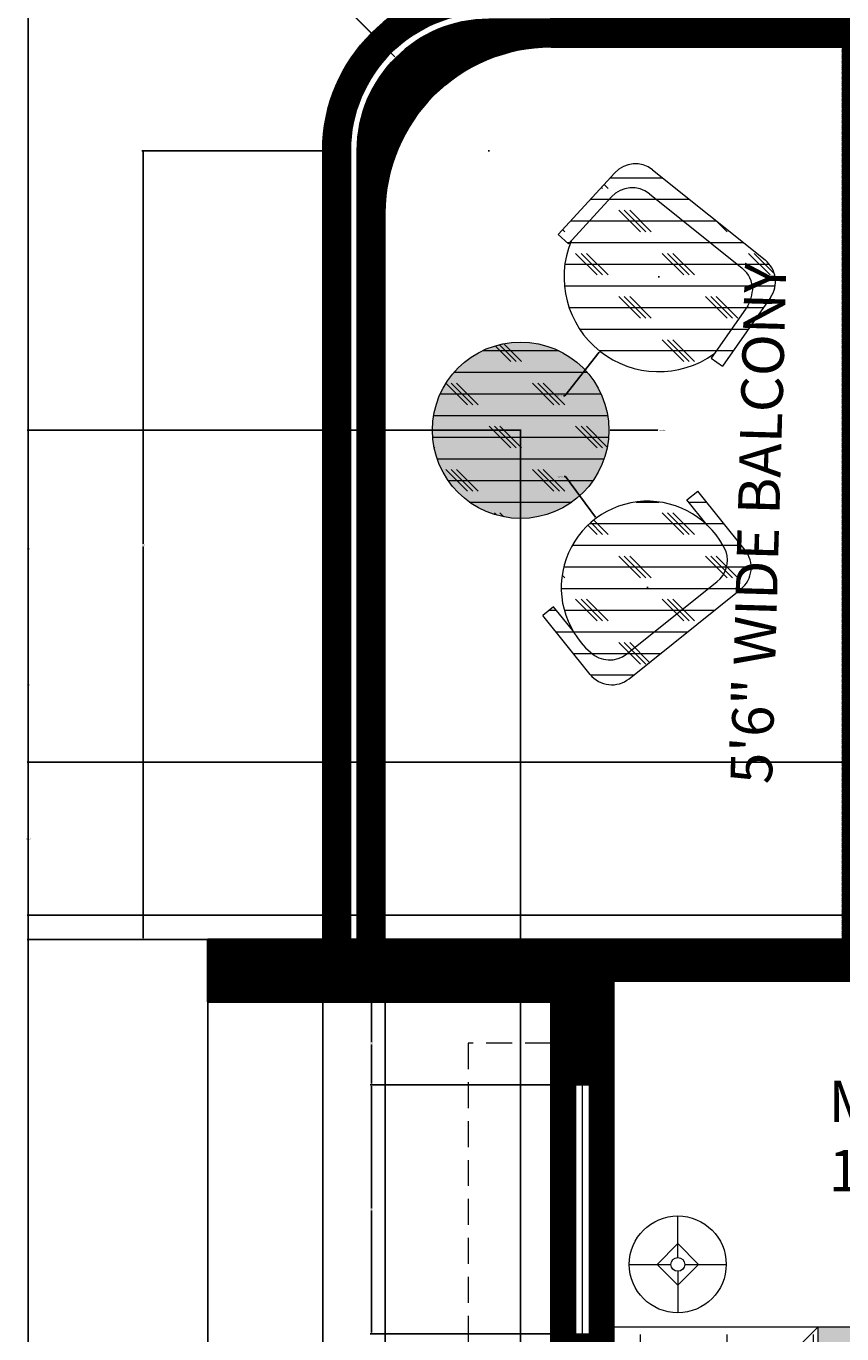
# Model space of a CAD drawing. Units: inches. Extents: x 557 to 1007, y 390 to 953.
# Tile 3 of 10: x 557 to 674, y 558 to 747. Entities that reach past the tile are written whole.
import ezdxf

# ---------------------------------------------------------------- set-up
doc = ezdxf.new("R2010")
doc.units = ezdxf.units.IN
doc.header["$LTSCALE"] = 5
doc.header["$MEASUREMENT"] = 0
doc.linetypes.add('HIDDEN', pattern=[0.375, 0.25, -0.125])
for name, color, linetype, lineweight in [('A-ANNO-DIMS', 2, 'Continuous', 18), ('A-AREA-IDEN', 7, 'Continuous', 18), ('A-FLOR-RAIL', 7, 'Continuous', 25), ('A-FURN', 8, 'Continuous', 18), ('A-FURN-PATT', 9, 'Continuous', 9), ('A-GLAZ', 4, 'Continuous', 18), ('A-GLAZ-OVHD', 8, 'HIDDEN', 13), ('A-WALL', 7, 'Continuous', 35), ('E-LITE', 2, 'Continuous', 13)]:
    doc.layers.add(name, color=color, linetype=linetype, lineweight=lineweight)
doc.layers.add('A-GLAZ-PATT', color=141, linetype='Continuous', lineweight=9, true_color=0xadddf7)
doc.layers.add('A-WALL-PATT', color=251, linetype='Continuous', lineweight=9, true_color=0x636466)
doc.styles.get("Standard").update_dxf_attribs({"font": 'arial.ttf'})
doc.dimstyles.get("Standard").update_dxf_attribs({"dimtxt": 0.18, "dimasz": 0.18, "dimexe": 0.18, "dimexo": 0.0625, "dimgap": 0.09, "dimtad": 0, "dimtih": 1, "dimtoh": 1, "dimdec": 4, "dimzin": 0, "dimdsep": 46, "dimtxsty": 'Standard', "dimcen": 0.09, "dimadec": 0, "dimazin": 0, "dimtfac": 1, "dimtdec": 4, "dimtofl": 0, "dimtmove": 0, "dimatfit": 3, "dimfxl": 1, "dimtolj": 1, "dimtzin": 0, "dimarcsym": 0})

# ---------------------------------------------------------------- blocks, each defined once
blk = doc.blocks.new('Lamp - Table')
for p, q in [((0, 7), (0, 1)), ((0, 3), (-3, 0)), ((3, 0), (0, 3)), ((-1, 0), (-7, 0)), ((-3, 0), (0, -3)), ((0, -3), (3, 0)), ((1, 0), (7, 0)), ((0, -1), (0, -7))]:
    blk.add_line(p, q)
for radius in [7, 1]:
    blk.add_circle((0, 0), radius)
blk = doc.blocks.new('BED-QUEEN-60x80-PLAN')
for p, q in [((0, 0), (0, 60)), ((0, 60), (80, 60)), ((29.6, 60), (14.4, 44.8)), ((29.6, 44.8), (29.6, 60)), ((80, 60), (80, 0)), ((1.2, 52), (16.4, 52)), ((1.2, 31.2), (1.2, 52)), ((16.4, 52), (16.4, 46.8)), ((14.4, 0), (14.4, 44.8)), ((14.4, 44.8), (29.6, 44.8)), ((16.8, 44.8), (16.8, 0)), ((14.4, 31.2), (1.2, 31.2)), ((1.2, 28.8), (14.4, 28.8)), ((1.2, 8), (1.2, 28.8)), ((14.4, 8), (1.2, 8)), ((80, 0), (0, 0))]:
    blk.add_line(p, q)
blk = doc.blocks.new('*D45')
at = {"layer": 'A-ANNO-DIMS', "color": 0, "lineweight": -2, "ltscale": 5, "transparency": 16777216}
for p, q in [((582.82, 605.84), (582.82, 389.77)), ((980.41, 439.84), (980.41, 389.77)), ((583, 389.95), (781.22, 389.95)), ((980.23, 389.95), (782.01, 389.95))]:
    blk.add_line(p, q, dxfattribs=at)
at = {"layer": 'A-ANNO-DIMS', "color": 0, "ltscale": 5, "transparency": 16777216}
for points in [[(583, 389.98), (583, 389.92), (582.82, 389.95)], [(980.23, 389.98), (980.23, 389.92), (980.41, 389.95)]]:
    blk.add_solid(points, dxfattribs=at)
at = {"layer": 'Defpoints', "color": 0, "ltscale": 5, "transparency": 16777216}
for p in [(582.82, 605.9), (980.41, 439.9), (980.41, 389.95)]:
    blk.add_point(p, dxfattribs=at)
at = {"layer": 'A-ANNO-DIMS', "color": 0, "ltscale": 5, "transparency": 16777216, "insert": (781.61, 389.95), "char_height": 0.18, "attachment_point": 5}
blk.add_mtext('\\A1;397.6', dxfattribs=at)
blk = doc.blocks.new('*D46')
at = {"layer": 'A-ANNO-DIMS', "color": 0, "lineweight": -2, "ltscale": 5, "transparency": 16777216}
for p, q in [((761.34, 926.9), (556.69, 926.9)), ((556.87, 926.72), (556.87, 671.59)), ((556.87, 416.08), (556.87, 671.22)), ((773.34, 415.9), (556.69, 415.9))]:
    blk.add_line(p, q, dxfattribs=at)
at = {"layer": 'A-ANNO-DIMS', "color": 0, "ltscale": 5, "transparency": 16777216}
for points in [[(556.84, 926.72), (556.9, 926.72), (556.87, 926.9)], [(556.84, 416.08), (556.9, 416.08), (556.87, 415.9)]]:
    blk.add_solid(points, dxfattribs=at)
at = {"layer": 'Defpoints', "color": 0, "ltscale": 5, "transparency": 16777216}
for p in [(556.87, 926.9), (761.41, 926.9), (773.41, 415.9)]:
    blk.add_point(p, dxfattribs=at)
at = {"layer": 'A-ANNO-DIMS', "color": 0, "ltscale": 5, "transparency": 16777216, "insert": (556.87, 671.4), "char_height": 0.18, "attachment_point": 5}
blk.add_mtext('\\A1;511', dxfattribs=at)
blk = doc.blocks.new('*D59')
at = {"layer": 'A-ANNO-DIMS', "color": 0, "lineweight": -2, "ltscale": 5, "transparency": 16777216}
for p, q in [((599.34, 728.9), (573.28, 728.9)), ((573.46, 728.72), (573.46, 672.08)), ((573.46, 615.08), (573.46, 671.72)), ((599.34, 614.9), (573.28, 614.9))]:
    blk.add_line(p, q, dxfattribs=at)
at = {"layer": 'A-ANNO-DIMS', "color": 0, "ltscale": 5, "transparency": 16777216}
for points in [[(573.43, 728.72), (573.49, 728.72), (573.46, 728.9)], [(573.43, 615.08), (573.49, 615.08), (573.46, 614.9)]]:
    blk.add_solid(points, dxfattribs=at)
at = {"layer": 'Defpoints', "color": 0, "ltscale": 5, "transparency": 16777216}
for p in [(573.46, 728.9), (599.41, 728.9), (599.41, 614.9)]:
    blk.add_point(p, dxfattribs=at)
at = {"layer": 'A-ANNO-DIMS', "color": 0, "ltscale": 5, "transparency": 16777216, "insert": (573.46, 671.9), "char_height": 0.18, "attachment_point": 5}
blk.add_mtext('\\A1;114', dxfattribs=at)
blk = doc.blocks.new('*D65')
at = {"layer": 'A-ANNO-DIMS', "color": 0, "lineweight": -2, "ltscale": 5, "transparency": 16777216}
for p, q in [((632.34, 593.9), (606.28, 593.9)), ((606.46, 593.72), (606.46, 576.09)), ((606.46, 558.08), (606.46, 575.72)), ((632.34, 557.9), (606.28, 557.9))]:
    blk.add_line(p, q, dxfattribs=at)
at = {"layer": 'A-ANNO-DIMS', "color": 0, "ltscale": 5, "transparency": 16777216}
for points in [[(606.43, 593.72), (606.49, 593.72), (606.46, 593.9)], [(606.43, 558.08), (606.49, 558.08), (606.46, 557.9)]]:
    blk.add_solid(points, dxfattribs=at)
at = {"layer": 'Defpoints', "color": 0, "ltscale": 5, "transparency": 16777216}
for p in [(606.46, 593.9), (632.41, 593.9), (632.41, 557.9)]:
    blk.add_point(p, dxfattribs=at)
at = {"layer": 'A-ANNO-DIMS', "color": 0, "ltscale": 5, "transparency": 16777216, "insert": (606.46, 575.9), "char_height": 0.18, "attachment_point": 5}
blk.add_mtext('\\A1;36', dxfattribs=at)
blk = doc.blocks.new('*D66')
at = {"layer": 'A-ANNO-DIMS', "color": 0, "lineweight": -2, "ltscale": 5, "transparency": 16777216}
for p, q in [((632.34, 605.9), (606.28, 605.9)), ((606.46, 605.72), (606.46, 600.08)), ((606.46, 594.08), (606.46, 599.72)), ((632.34, 593.9), (606.28, 593.9))]:
    blk.add_line(p, q, dxfattribs=at)
at = {"layer": 'A-ANNO-DIMS', "color": 0, "ltscale": 5, "transparency": 16777216}
for points in [[(606.43, 605.72), (606.49, 605.72), (606.46, 605.9)], [(606.43, 594.08), (606.49, 594.08), (606.46, 593.9)]]:
    blk.add_solid(points, dxfattribs=at)
at = {"layer": 'Defpoints', "color": 0, "ltscale": 5, "transparency": 16777216}
for p in [(606.46, 605.9), (632.41, 605.9), (632.41, 593.9)]:
    blk.add_point(p, dxfattribs=at)
at = {"layer": 'A-ANNO-DIMS', "color": 0, "ltscale": 5, "transparency": 16777216, "insert": (606.46, 599.9), "char_height": 0.18, "attachment_point": 5}
blk.add_mtext('\\A1;12', dxfattribs=at)
blk = doc.blocks.new('*D75')
at = {"layer": 'A-ANNO-DIMS', "color": 0, "lineweight": -2, "ltscale": 5, "transparency": 16777216}
for p, q in [((582.82, 614.84), (582.82, 389.77)), ((599.41, 614.84), (599.41, 389.77)), ((583, 389.95), (590.66, 389.95)), ((599.23, 389.95), (591.57, 389.95))]:
    blk.add_line(p, q, dxfattribs=at)
at = {"layer": 'A-ANNO-DIMS', "color": 0, "ltscale": 5, "transparency": 16777216}
for points in [[(583, 389.98), (583, 389.92), (582.82, 389.95)], [(599.23, 389.98), (599.23, 389.92), (599.41, 389.95)]]:
    blk.add_solid(points, dxfattribs=at)
at = {"layer": 'Defpoints', "color": 0, "ltscale": 5, "transparency": 16777216}
for p in [(582.82, 614.9), (599.41, 614.9), (582.82, 389.95)]:
    blk.add_point(p, dxfattribs=at)
at = {"layer": 'A-ANNO-DIMS', "color": 0, "ltscale": 5, "transparency": 16777216, "insert": (591.11, 389.95), "char_height": 0.18, "attachment_point": 5}
blk.add_mtext('\\A1;16.582', dxfattribs=at)
blk = doc.blocks.new('*D81')
at = {"layer": 'A-ANNO-DIMS', "color": 0, "lineweight": -2, "ltscale": 5, "transparency": 16777216}
for p, q in [((874.87, 640.54), (556.69, 640.54)), ((556.87, 640.36), (556.87, 629.66)), ((556.87, 618.59), (556.87, 629.29)), ((870.87, 618.41), (556.69, 618.41))]:
    blk.add_line(p, q, dxfattribs=at)
at = {"layer": 'A-ANNO-DIMS', "color": 0, "ltscale": 5, "transparency": 16777216}
for points in [[(556.84, 640.36), (556.9, 640.36), (556.87, 640.54)], [(556.84, 618.59), (556.9, 618.59), (556.87, 618.41)]]:
    blk.add_solid(points, dxfattribs=at)
at = {"layer": 'Defpoints', "color": 0, "ltscale": 5, "transparency": 16777216}
for p in [(874.93, 640.54), (556.87, 618.41), (870.93, 618.41)]:
    blk.add_point(p, dxfattribs=at)
at = {"layer": 'A-ANNO-DIMS', "color": 0, "ltscale": 5, "transparency": 16777216, "insert": (556.87, 629.48), "char_height": 0.18, "attachment_point": 5}
blk.add_mtext('\\A1;22.13', dxfattribs=at)
blk = doc.blocks.new('*D91')
at = {"layer": 'A-ANNO-DIMS', "color": 0, "lineweight": -2, "ltscale": 5, "transparency": 16777216}
for p, q in [((628, 688.44), (628, 389.77)), ((608.41, 614.84), (608.41, 389.77)), ((608.59, 389.95), (617.75, 389.95)), ((627.82, 389.95), (618.66, 389.95))]:
    blk.add_line(p, q, dxfattribs=at)
at = {"layer": 'A-ANNO-DIMS', "color": 0, "ltscale": 5, "transparency": 16777216}
for points in [[(608.59, 389.98), (608.59, 389.92), (608.41, 389.95)], [(627.82, 389.98), (627.82, 389.92), (628, 389.95)]]:
    blk.add_solid(points, dxfattribs=at)
at = {"layer": 'Defpoints', "color": 0, "ltscale": 5, "transparency": 16777216}
for p in [(628, 688.5), (608.41, 614.9), (608.41, 389.95)]:
    blk.add_point(p, dxfattribs=at)
at = {"layer": 'A-ANNO-DIMS', "color": 0, "ltscale": 5, "transparency": 16777216, "insert": (618.2, 389.95), "char_height": 0.18, "attachment_point": 5}
blk.add_mtext('\\A1;19.595', dxfattribs=at)
blk = doc.blocks.new('*D92')
at = {"layer": 'A-ANNO-DIMS', "color": 0, "lineweight": -2, "ltscale": 5, "transparency": 16777216}
for p, q in [((627.94, 688.5), (556.69, 688.5)), ((556.87, 688.32), (556.87, 651.88)), ((556.87, 615.08), (556.87, 651.52)), ((608.34, 614.9), (556.69, 614.9))]:
    blk.add_line(p, q, dxfattribs=at)
at = {"layer": 'A-ANNO-DIMS', "color": 0, "ltscale": 5, "transparency": 16777216}
for points in [[(556.84, 688.32), (556.9, 688.32), (556.87, 688.5)], [(556.84, 615.08), (556.9, 615.08), (556.87, 614.9)]]:
    blk.add_solid(points, dxfattribs=at)
at = {"layer": 'Defpoints', "color": 0, "ltscale": 5, "transparency": 16777216}
for p in [(628, 688.5), (556.87, 614.9), (608.41, 614.9)]:
    blk.add_point(p, dxfattribs=at)
at = {"layer": 'A-ANNO-DIMS', "color": 0, "ltscale": 5, "transparency": 16777216, "insert": (556.87, 651.7), "char_height": 0.18, "attachment_point": 5}
blk.add_mtext('\\A1;73.6', dxfattribs=at)
blk = doc.blocks.new('*D101')
at = {"layer": 'A-ANNO-DIMS', "color": 0, "lineweight": -2, "ltscale": 5, "transparency": 16777216}
for p, q in [((596.07, 756.06), (596.25, 756.06)), ((596.25, 756.06), (606.31, 746)), ((623.32, 728.9), (623.5, 728.9)), ((623.41, 728.81), (623.41, 728.99))]:
    blk.add_line(p, q, dxfattribs=at)
at = {"layer": 'A-ANNO-DIMS', "color": 0, "ltscale": 5, "transparency": 16777216}
blk.add_solid([(606.33, 746.02), (606.29, 745.98), (606.43, 745.88)], dxfattribs=at)
at = {"layer": 'Defpoints', "color": 0, "ltscale": 5, "transparency": 16777216}
for p in [(606.43, 745.88), (623.41, 728.9)]:
    blk.add_point(p, dxfattribs=at)
at = {"layer": 'A-ANNO-DIMS', "color": 0, "ltscale": 5, "transparency": 16777216, "insert": (595.57, 756.06), "char_height": 0.18, "attachment_point": 5}
blk.add_mtext('\\A1;2X R24', dxfattribs=at)
blk = doc.blocks.new('*D102')
at = {"layer": 'A-ANNO-DIMS', "color": 0, "lineweight": -2, "ltscale": 5, "transparency": 16777216}
for p, q in [((600.6, 751.53), (600.78, 751.53)), ((600.78, 751.53), (609.14, 743.17)), ((623.32, 728.9), (623.5, 728.9)), ((623.41, 728.81), (623.41, 728.99))]:
    blk.add_line(p, q, dxfattribs=at)
at = {"layer": 'A-ANNO-DIMS', "color": 0, "ltscale": 5, "transparency": 16777216}
blk.add_solid([(609.16, 743.2), (609.11, 743.15), (609.26, 743.05)], dxfattribs=at)
at = {"layer": 'Defpoints', "color": 0, "ltscale": 5, "transparency": 16777216}
for p in [(609.26, 743.05), (623.41, 728.9)]:
    blk.add_point(p, dxfattribs=at)
at = {"layer": 'A-ANNO-DIMS', "color": 0, "ltscale": 5, "transparency": 16777216, "insert": (600.29, 751.53), "char_height": 0.18, "attachment_point": 5}
blk.add_mtext('\\A1;R20', dxfattribs=at)
blk = doc.blocks.new('*D103')
at = {"layer": 'A-ANNO-DIMS', "color": 0, "lineweight": -2, "ltscale": 5, "transparency": 16777216}
for p, q in [((601.73, 750.4), (601.91, 750.4)), ((601.91, 750.4), (609.84, 742.47)), ((623.32, 728.9), (623.5, 728.9)), ((623.41, 728.81), (623.41, 728.99))]:
    blk.add_line(p, q, dxfattribs=at)
at = {"layer": 'A-ANNO-DIMS', "color": 0, "ltscale": 5, "transparency": 16777216}
blk.add_solid([(609.86, 742.49), (609.82, 742.45), (609.97, 742.34)], dxfattribs=at)
at = {"layer": 'Defpoints', "color": 0, "ltscale": 5, "transparency": 16777216}
for p in [(609.97, 742.34), (623.41, 728.9)]:
    blk.add_point(p, dxfattribs=at)
at = {"layer": 'A-ANNO-DIMS', "color": 0, "ltscale": 5, "transparency": 16777216, "insert": (601.42, 750.4), "char_height": 0.18, "attachment_point": 5}
blk.add_mtext('\\A1;R19', dxfattribs=at)
blk = doc.blocks.new('*D104')
at = {"layer": 'A-ANNO-DIMS', "color": 0, "lineweight": -2, "ltscale": 5, "transparency": 16777216}
for p, q in [((627.91, 688.5), (628.09, 688.5)), ((628, 688.41), (628, 688.59)), ((647.83, 688.5), (640.93, 688.5))]:
    blk.add_line(p, q, dxfattribs=at)
at = {"layer": 'A-ANNO-DIMS', "color": 0, "ltscale": 5, "transparency": 16777216}
blk.add_solid([(640.93, 688.53), (640.93, 688.47), (640.75, 688.5)], dxfattribs=at)
at = {"layer": 'Defpoints', "color": 0, "ltscale": 5, "transparency": 16777216}
for p in [(615.25, 688.5), (640.75, 688.5)]:
    blk.add_point(p, dxfattribs=at)
at = {"layer": 'A-ANNO-DIMS', "color": 0, "ltscale": 5, "transparency": 16777216, "insert": (648.4, 688.5), "char_height": 0.18, "attachment_point": 5}
blk.add_mtext('\\A1;∅25.495', dxfattribs=at)
blk = doc.blocks.new('*D114')
at = {"layer": 'A-ANNO-DIMS', "color": 0, "lineweight": -2, "ltscale": 5, "transparency": 16777216}
for p, q in [((647.87, 710.66), (648.05, 710.66)), ((647.96, 710.57), (647.96, 710.75)), ((634.37, 693.48), (639.36, 699.78)), ((634.19, 693.48), (634.37, 693.48))]:
    blk.add_line(p, q, dxfattribs=at)
at = {"layer": 'A-ANNO-DIMS', "color": 0, "ltscale": 5, "transparency": 16777216}
blk.add_solid([(639.33, 699.8), (639.38, 699.76), (639.47, 699.92)], dxfattribs=at)
at = {"layer": 'Defpoints', "color": 0, "ltscale": 5, "transparency": 16777216}
for p in [(647.96, 710.66), (639.47, 699.92)]:
    blk.add_point(p, dxfattribs=at)
at = {"layer": 'A-ANNO-DIMS', "color": 0, "ltscale": 5, "transparency": 16777216, "insert": (633.51, 693.48), "char_height": 0.18, "attachment_point": 5}
blk.add_mtext('\\A1;2X R13.69', dxfattribs=at)
blk = doc.blocks.new('*D115')
at = {"layer": 'A-ANNO-DIMS', "color": 0, "lineweight": -2, "ltscale": 5, "transparency": 16777216}
for p, q in [((634.28, 681.8), (634.46, 681.8)), ((634.46, 681.8), (638.81, 675.93)), ((646.26, 665.76), (646.44, 665.76)), ((646.35, 665.67), (646.35, 665.85))]:
    blk.add_line(p, q, dxfattribs=at)
at = {"layer": 'A-ANNO-DIMS', "color": 0, "ltscale": 5, "transparency": 16777216}
blk.add_solid([(638.83, 675.95), (638.79, 675.91), (638.92, 675.79)], dxfattribs=at)
at = {"layer": 'Defpoints', "color": 0, "ltscale": 5, "transparency": 16777216}
for p in [(638.92, 675.79), (646.35, 665.76)]:
    blk.add_point(p, dxfattribs=at)
at = {"layer": 'A-ANNO-DIMS', "color": 0, "ltscale": 5, "transparency": 16777216, "insert": (633.73, 681.8), "char_height": 0.18, "attachment_point": 5}
blk.add_mtext('\\A1;R12.476', dxfattribs=at)

msp = doc.modelspace()

# ---------------------------------------------------------------- hatches: boundary and pattern name
at = {"layer": 'A-FURN-PATT', "ltscale": 5}
h = msp.add_hatch(dxfattribs=at)
h.set_pattern_fill('GRAVEL', color=256, scale=25)
h.set_pattern_definition([(228.01279, (18, 25), (-200, -225), [3.3634, -332.9772]), (184.96974, (15.75, 22.5), (300, 25), [5.7717, -571.39812]), (132.51045, (10, 22), (250, -275), [4.0697, -402.9008]), (267.27369, (0.25, 15.75), (25, 500), [5.25595, -520.33895]), (292.83365, (0, 10.5), (-125, 300), [5.15387, -510.23433]), (357.27369, (2, 5.75), (-500, 25), [5.25595, -520.33895]), (37.69424, (7.25, 5.5), (-325, -250), [6.95072, -688.1212]), (72.25533, (12.75, 9.75), (175, 550), [6.5622, -649.65804]), (121.42957, (14.75, 16), (-200, 325), [5.27375, -522.10183]), (175.23636, (12, 20.5), (275, -25), [6.0208, -295.01906]), (222.39744, (6, 21), (-300, -275), [7.7862, -770.83438]), (138.81407, (25, 15.5), (-175, 150), [2.65752, -263.0961]), (171.46923, (23, 17.25), (325, -50), [5.05593, -500.5378]), (225, (18, 18), (-3e-15, -25), [3.53552, -31.8198]), (203.1986, (16.25, 21), (125, 50), [1.90395, -188.49038]), (291.8014, (14.5, 20.25), (-25, 75), [2.69257, -131.93655]), (30.96376, (15.5, 17.75), (75, 50), [4.37322, -141.40057]), (161.56505, (19.25, 20), (50, -25), [3.16228, -75.89467]), (16.38954, (0, 20.25), (250, 75), [4.43, -438.57113]), (70.34618, (4.25, 21.5), (-100, -275), [3.71652, -367.9352]), (293.1986, (19.25, 25), (-50, 125), [3.80788, -186.58645]), (343.61046, (20.75, 21.5), (-250, 75), [4.43, -438.57113]), (339.44395, (0, 4.75), (-125, 50), [4.272, -209.3281]), (294.77514, (4, 3.25), (-125, 275), [3.57945, -354.36608]), (66.8014, (19.5, 0), (50, 125), [3.80788, -186.58645]), (17.35402, (21, 3.5), (-325, -100), [4.19078, -414.8856]), (69.44395, (7.25, 0), (-50, -125), [2.136, -211.4641]), (101.30993, (18, 0), (-25, 100), [1.27475, -126.20074]), (165.96376, (17.75, 1.25), (75, -25), [5.15388, -97.92377]), (186.00901, (12.75, 2.5), (250, 25), [4.77625, -472.84808]), (303.69007, (15.5, 15.5), (-25, 50), [3.60555, -86.53323]), (353.15723, (17.5, 12.5), (425, -50), [6.29485, -623.18907]), (60.9454, (23.75, 11.75), (-100, -175), [2.5739, -254.81685]), (90, (25, 14), (-25, 25), [1.5, -23.5]), (120.25644, (12.25, 3.25), (100, -175), [3.4731, -343.838]), (48.01279, (10.5, 6.25), (200, 225), [6.7268, -329.6138]), (0, (15, 11.25), (25, 25), [6.5, -18.5]), (325.30485, (21.5, 11.25), (250, -175), [3.95285, -391.33186]), (254.0546, (24.75, 9), (-25, -100), [3.64005, -178.3627]), (207.64598, (23.75, 5.5), (-475, -250), [5.92662, -586.73685]), (175.42608, (18.5, 2.75), (-325, 25), [6.26997, -620.72684])])
h.paths.add_polyline_path([(615.2525, 688.5, 1), (640.7475, 688.5, 1)])
h.paths.add_polyline_path([(917.0544, 663.8414, 0.33333323), (915.2241, 665.6717), (882.2793, 665.6717, 0.33333323), (880.449, 663.8414), (880.449, 649.1992, 0.33333323), (882.2793, 647.369), (915.2241, 647.369, 0.33333323), (917.0544, 649.1992)])
h.paths.add_polyline_path([(828.0807, 699.7098), (756.0807, 699.7098), (756.0807, 663.7098), (828.0807, 663.7098)])
h.paths.add_polyline_path([(787.5651, 663.7098), (768.5964, 663.7098), (769.8463, 655.7098), (786.3151, 655.7098)])
h.paths.add_polyline_path([(815.5651, 663.7098), (796.5964, 663.7098), (797.8463, 655.7098), (814.3151, 655.7098)])
h.paths.add_polyline_path([(836.0807, 689.9442), (828.0807, 691.1942), (828.0807, 672.2255), (836.0807, 673.4755)])
h.paths.add_polyline_path([(756.0807, 691.1942), (748.0807, 689.9442), (748.0807, 673.4755), (756.0807, 672.2255)])
h.paths.add_polyline_path([(786.3151, 707.7098), (769.8463, 707.7098), (768.5964, 699.7098), (787.5651, 699.7098)])
h.paths.add_polyline_path([(814.3151, 707.7098), (797.8463, 707.7098), (796.5964, 699.7098), (815.5651, 699.7098)])
h.paths.add_polyline_path([(917.4362, 607.3575), (889.5896, 607.3575), (889.5896, 586.4726), (917.4362, 586.4726)])
h.paths.add_polyline_path([(721.4053, 881.8539), (671.0053, 881.8539), (671.0053, 866.6539), (658.2053, 866.6539), (658.2053, 821.8539), (721.4053, 821.8539)])
h.paths.add_polyline_path([(925.4053, 875.1046), (875.0053, 875.1046), (875.0053, 859.9046), (862.2053, 859.9046), (862.2053, 815.1046), (925.4053, 815.1046)])
h.paths.add_polyline_path([(721.4053, 558.9046), (671.0053, 558.9046), (671.0053, 543.7046), (658.2053, 543.7046), (658.2053, 498.9046), (721.4053, 498.9046)])
at = {"layer": 'A-FURN-PATT'}
h = msp.add_hatch(dxfattribs=at)
h.set_pattern_fill('CROSS', color=256, scale=25)
h.paths.add_polyline_path([(925.4053, 875.1046), (875.0053, 875.1046), (875.0053, 859.9046), (862.2053, 859.9046), (862.2053, 815.1046), (925.4053, 815.1046)])
h.paths.add_polyline_path([(721.4053, 881.8539), (671.0053, 881.8539), (671.0053, 866.6539), (658.2053, 866.6539), (658.2053, 821.8539), (721.4053, 821.8539)])
h.paths.add_polyline_path([(671.0053, 881.8539), (655.8053, 866.6539), (671.0053, 866.6539)], flags=17)
h.paths.add_polyline_path([(671.0053, 881.8539), (641.4053, 881.8539), (641.4053, 821.8539), (655.8053, 821.8539), (655.8053, 829.8539), (642.6053, 829.8539), (642.6053, 850.6539), (655.8053, 850.6539), (655.8053, 853.0539), (642.6053, 853.0539), (642.6053, 873.8539), (657.8053, 873.8539), (657.8053, 868.6539)])
h.paths.add_polyline_path([(875.0053, 875.1046), (859.8053, 859.9046), (875.0053, 859.9046)], flags=17)
h.paths.add_polyline_path([(875.0053, 875.1046), (845.4053, 875.1046), (845.4053, 815.1046), (859.8053, 815.1046), (859.8053, 823.1046), (846.6053, 823.1046), (846.6053, 843.9046), (859.8053, 843.9046), (859.8053, 846.3046), (846.6053, 846.3046), (846.6053, 867.1046), (861.8053, 867.1046), (861.8053, 861.9046)])
h.paths.add_polyline_path([(721.4053, 558.9046), (671.0053, 558.9046), (671.0053, 543.7046), (658.2053, 543.7046), (658.2053, 498.9046), (721.4053, 498.9046)])
h.paths.add_polyline_path([(671.0053, 558.9046), (641.4053, 558.9046), (641.4053, 498.9046), (655.8053, 498.9046), (655.8053, 506.9046), (642.6053, 506.9046), (642.6053, 527.7046), (655.8053, 527.7046), (655.8053, 530.1046), (642.6053, 530.1046), (642.6053, 550.9046), (657.8053, 550.9046), (657.8053, 545.7046)])
h.paths.add_polyline_path([(671.0053, 558.9046), (657.8053, 545.7046), (655.8053, 543.7046), (671.0053, 543.7046)], flags=17)
h.paths.add_polyline_path([(873.1461, 661.8773, 0.41421356), (868.1461, 666.8773, -0.12244426), (867.1516, 666.8773), (855.014, 666.8773), (855.014, 647.2429), (867.4581, 647.2429, -0.08537395), (868.1461, 647.2429, 0.41421356), (873.1461, 652.2429)])
h.paths.add_polyline_path([(917.0544, 663.8414, 0.33333323), (915.2241, 665.6717), (882.2793, 665.6717, 0.33333323), (880.449, 663.8414), (880.449, 649.1992, 0.33333323), (882.2793, 647.369), (915.2241, 647.369, 0.33333323), (917.0544, 649.1992)])
h.paths.add_polyline_path([(944.9465, 667.5202), (932.6561, 667.5202, -0.10407786), (931.8144, 667.5202, 0.41421356), (926.8144, 662.5202), (926.8144, 652.8858, 0.41421356), (931.8144, 647.8858, -0.05611627), (932.2647, 647.8858), (944.9465, 647.8858)])
h.paths.add_polyline_path([(928.8341, 635.542, 0.41421356), (923.8341, 640.542), (914.1997, 640.542, 0.41421356), (909.1997, 635.542), (909.1997, 622.4099), (923.8341, 622.4099, 0.41421356), (928.8341, 627.4099)])
h.paths.add_polyline_path([(909.1997, 635.542, 0.41421356), (904.1997, 640.542), (894.5653, 640.542, 0.41421356), (889.5653, 635.542), (889.5653, 622.4099), (909.1997, 622.4099)])
h.paths.add_polyline_path([(889.5653, 635.542, 0.41421356), (884.5653, 640.542), (874.9308, 640.542, 0.41421356), (869.9308, 635.542), (869.9308, 627.4099, 0.41421356), (874.9308, 622.4099), (889.5653, 622.4099)])
h = msp.add_hatch(dxfattribs=at)
h.set_pattern_fill('CORK', color=256, scale=25)
h.set_pattern_definition([(0, (0, 0), (0, 3.125), []), (135, (1.5625, -1.5625), (-6.25, -6.25), [4.41942, -4.41942]), (135, (2.344, -1.5625), (-6.25, -6.25), [4.41942, -4.41942]), (135, (3.125, -1.5625), (-6.25, -6.25), [4.41942, -4.41942])])
h.paths.add_polyline_path([(932.8341, 623.4099), (932.8341, 630.9869, 0.76666915), (928.8341, 630.9869), (928.8341, 627.4099), (928.8341, 622.4099), (909.1997, 622.4099), (874.9308, 622.4099), (869.9308, 622.4099), (869.9308, 632.3614, 0.60407544), (865.9308, 632.3614), (865.9308, 623.4099, 0.41421356), (870.9308, 618.4099), (927.8341, 618.4099, 0.41421356)])
h.paths.add_polyline_path([(855.014, 666.8773), (868.1461, 666.8773, 0.78182568), (868.1461, 670.8773), (855.014, 670.8773, 0.41421356), (850.014, 665.8773), (850.014, 648.2429, 0.41421356), (855.014, 643.2429), (868.1461, 643.2429, 0.84268288), (868.1461, 647.2429), (855.014, 647.2429)])
h.paths.add_polyline_path([(948.9465, 666.5202, 0.41421356), (943.9465, 671.5202), (931.8144, 671.5202, 0.81146646), (931.8144, 667.5202), (944.9465, 667.5202), (944.9465, 647.8858), (931.8144, 647.8858, 0.89373088), (931.8144, 643.8858), (943.9465, 643.8858, 0.41421356), (948.9465, 648.8858)])
h.paths.add_polyline_path([(951.6399, 638.9424), (935.2317, 638.9424), (935.2317, 622.9231), (951.6399, 622.9231)])
h.paths.add_polyline_path([(947.0475, 626.5028), (947.0441, 626.4915), (947.0523, 626.4868)], flags=16)
h.paths.add_polyline_path([(944.6349, 630.5579), (944.0837, 633.55), (944.1177, 633.5282), (944.0932, 633.4983), (944.6349, 630.5579), (947.5056, 631.5148), (947.5212, 631.5348), (947.5189, 631.5192), (944.6349, 630.5579), (944.8619, 630.2742), (944.9055, 630.2607), (944.8981, 630.2289)], flags=16)
h.paths.add_polyline_path([(863.4458, 638.9424), (847.0376, 638.9424), (847.0376, 622.9231), (863.4458, 622.9231)])
h.paths.add_polyline_path([(858.2228, 627.4003), (858.2193, 627.3889), (858.2276, 627.3842)], flags=16)
h.paths.add_polyline_path([(855.8101, 631.4553), (855.259, 634.4474), (855.2929, 634.4257), (855.2685, 634.3958), (855.8101, 631.4553), (858.6808, 632.4122), (858.6964, 632.4323), (858.6941, 632.4166), (855.8101, 631.4553), (856.0371, 631.1716), (856.0807, 631.1581), (856.0733, 631.1263)], flags=16)
h.paths.add_polyline_path([(638.0774, 656.4227, 0.37705983), (643.354, 656.1836), (656.3799, 666.6283, 0.31001778), (657.6899, 670.9599, 1.23353517)], flags=17)
h.paths.add_polyline_path([(659.8169, 665.539, 0.41421356), (660.4353, 671.1619), (653.5962, 679.6912), (652.0359, 678.44), (654.9689, 674.7822, -0.09486374), (657.6899, 670.9599, -0.31001778), (656.3799, 666.6283), (643.354, 656.1836, -0.37705983), (638.0774, 656.4227, -0.08126294), (635.5314, 659.5452), (632.7686, 662.9907), (631.2083, 661.7396), (638.0474, 653.2104, 0.41421356), (643.6703, 652.592)])
h.paths.add_polyline_path([(646.6056, 722.6678, 0.39517975), (641.1529, 722.2481), (635.2941, 715.8481, 0.75247437), (655.9256, 699.5214), (660.8023, 706.4923, 0.05595903), (661.2292, 707.2762, 0.02810216), (661.5248, 708.7853, 0.22754294), (660.027, 711.9059)])
h.paths.add_polyline_path([(647.072, 726.1392, 0.39517975), (641.6193, 725.7194), (633.4395, 716.7841), (634.9147, 715.4336), (641.1529, 722.2481, -0.39517975), (646.6056, 722.6678), (660.027, 711.9059, -0.22754294), (661.5248, 708.7853, -0.02810216), (661.2292, 707.2762, -0.05595903), (660.8023, 706.4923), (655.9256, 699.5214), (655.5065, 698.9223), (657.1453, 697.7758), (664.0894, 707.702, 0.39517975), (663.3141, 713.1156)])
h.paths.add_polyline_path([(640.7475, 688.5, 1), (615.2525, 688.5, 1)])
at = {"layer": 'A-GLAZ-PATT'}
h = msp.add_hatch(dxfattribs=at)
h.set_pattern_fill('ANSI31', color=256)
h.paths.add_polyline_path([(635.9053, 814.7688), (636.9053, 814.7688), (636.9053, 838.7688), (632.4053, 838.7688), (632.4053, 790.7688), (635.9053, 790.7688)])
h.paths.add_polyline_path([(641.4053, 838.7688), (637.9053, 838.7688), (637.9053, 814.7688), (636.9053, 814.7688), (636.9053, 790.7688), (641.4053, 790.7688)])
h.paths.add_polyline_path([(603.4053, 728.9046, -0.41421356), (623.4053, 748.9046), (632.4053, 748.9046), (632.4053, 752.9046), (623.4053, 752.9046, 0.41421356), (599.4053, 728.9046), (599.4053, 614.9046), (603.4053, 614.9046)])
h.paths.add_polyline_path([(632.4053, 743.9046), (632.4053, 747.9046), (623.4053, 747.9046, 0.41421356), (604.4053, 728.9046), (604.4053, 614.9046), (608.4053, 614.9046), (608.4053, 719.9046, -0.41421356)])
h.paths.add_polyline_path([(683.4053, 722.9046), (678.9053, 722.9046), (678.9053, 698.9046), (679.9053, 698.9046), (679.9053, 662.9046), (678.9053, 662.9046), (678.9053, 638.9046), (683.4053, 638.9046)])
h.paths.add_polyline_path([(678.9053, 698.9046), (677.9053, 698.9046), (677.9053, 722.9046), (674.4053, 722.9046), (674.4053, 638.9046), (677.9053, 638.9046), (677.9053, 662.9046), (678.9053, 662.9046)])
h.paths.add_polyline_path([(635.9053, 593.9046), (632.4053, 593.9046), (632.4053, 557.9046), (635.9053, 557.9046)])
h.paths.add_polyline_path([(641.4053, 593.9046), (637.9053, 593.9046), (637.9053, 557.9046), (641.4053, 557.9046)])
h.paths.add_polyline_path([(764.9579, 448.9046), (716.9579, 448.9046), (716.9579, 445.4046), (740.9579, 445.4046), (740.9579, 444.4046), (764.9579, 444.4046)])
h.paths.add_polyline_path([(764.9579, 443.4046), (740.9579, 443.4046), (740.9579, 444.4046), (716.9579, 444.4046), (716.9579, 439.9046), (764.9579, 439.9046)])
h.paths.add_polyline_path([(938.4053, 905.9046), (878.4053, 905.9046), (878.4053, 902.4046), (908.4053, 902.4046), (908.4053, 901.4046), (938.4053, 901.4046)])
h.paths.add_polyline_path([(938.4053, 900.4046), (908.4053, 900.4046), (908.4053, 901.4046), (878.4053, 901.4046), (878.4053, 896.9046), (938.4053, 896.9046)])
h.paths.add_polyline_path([(724.9087, 905.9046), (676.9087, 905.9046), (676.9087, 902.4046), (701.4053, 902.4046), (701.4053, 901.4046), (724.9087, 901.4046)])
h.paths.add_polyline_path([(724.9087, 900.4046), (701.4053, 900.4046), (701.4053, 901.4046), (676.9087, 901.4046), (676.9087, 896.9046), (724.9087, 896.9046)])
h.paths.add_polyline_path([(832.0625, 905.9046), (808.0625, 905.9046), (808.0625, 902.4046), (832.0625, 902.4046)])
h.paths.add_polyline_path([(832.0625, 900.4046), (808.0625, 900.4046), (808.0625, 896.9046), (832.0625, 896.9046)])
at = {"layer": 'A-WALL-PATT'}
h = msp.add_hatch(dxfattribs=at)
h.set_pattern_fill('ANSI31', color=256)
h.paths.add_polyline_path([(808.0625, 905.9046), (767.4053, 905.9046), (767.4053, 920.9046), (839.4053, 920.9046), (839.4053, 905.9046), (832.0625, 905.9046), (832.0625, 896.9046), (839.4053, 896.9046), (839.4053, 800.9046), (837.4053, 800.9046), (837.4053, 794.9046), (839.4053, 794.9046), (839.4053, 790.9046), (845.4053, 790.9046), (845.4053, 896.9046), (878.4053, 896.9046), (878.4053, 905.9046), (845.4053, 905.9046), (845.4053, 926.9046), (761.4053, 926.9046), (761.4053, 914.9046), (761.4053, 905.9046), (724.9087, 905.9046), (724.9087, 896.9046), (761.4053, 896.9046), (761.4053, 752.9046), (759.4053, 752.9046), (759.4053, 746.9046), (767.4053, 746.9046), (767.4053, 794.9046), (807.4053, 794.9046), (807.4053, 800.9046), (767.4053, 800.9046), (767.4053, 896.9046), (808.0625, 896.9046)])
h.paths.add_polyline_path([(676.9087, 905.9046), (632.4053, 905.9046), (632.4053, 838.7688), (641.4053, 838.7688), (641.4053, 881.8539), (641.4053, 896.9046), (676.9087, 896.9046)])
h.paths.add_polyline_path([(980.4053, 905.9046), (938.4053, 905.9046), (938.4053, 896.9046), (971.4053, 896.9046), (971.4053, 752.9046), (845.4053, 752.9046), (845.4053, 754.9046), (839.4053, 754.9046), (839.4053, 746.9046), (971.4053, 746.9046), (971.4053, 720.1788), (980.4053, 720.1788)])
h.paths.add_polyline_path([(723.4053, 752.9046), (641.4053, 752.9046), (641.4053, 790.7688), (632.4053, 790.7688), (632.4053, 743.9046), (674.4053, 743.9046), (674.4053, 722.9046), (683.4053, 722.9046), (683.4053, 746.9046), (723.4053, 746.9046)])
h.paths.add_polyline_path([(980.4053, 684.1788), (971.4053, 684.1788), (971.4053, 614.9046), (845.4053, 614.9046), (845.4053, 608.9046), (971.4053, 608.9046), (971.4053, 512.9046), (908.7697, 512.9046), (908.7697, 508.9046), (971.4053, 508.9046), (971.4053, 448.9046), (845.4053, 448.9046), (845.4053, 508.9046), (878.7697, 508.9046), (878.7697, 512.9046), (845.4053, 512.9046), (845.4053, 562.9046), (779.4053, 562.9046), (779.4053, 614.9046), (761.4053, 614.9046), (761.4053, 608.9046), (773.4053, 608.9046), (773.4053, 512.636), (779.4053, 512.636), (779.4053, 556.9046), (839.4053, 556.9046), (839.4053, 448.9046), (830.432, 448.9046), (830.432, 439.9046), (839.4053, 439.9046), (839.4053, 433.0506), (839.4053, 421.9046), (779.4053, 421.9046), (779.4053, 439.9046), (796.9656, 439.9046), (806.432, 439.9046), (806.432, 448.9046), (779.4053, 448.9046), (779.4053, 482.636), (773.4053, 482.636), (773.4053, 448.9046), (764.9579, 448.9046), (764.9579, 439.9046), (773.4053, 439.9046), (773.4053, 415.9046), (845.4053, 415.9046), (845.4053, 439.9046), (980.4053, 439.9046)])
h.paths.add_polyline_path([(716.9579, 448.9046), (641.4053, 448.9046), (641.4053, 557.9046), (632.4053, 557.9046), (632.4053, 439.9046), (716.9579, 439.9046)])
h.paths.add_polyline_path([(725.4053, 614.9046), (683.4053, 614.9046), (683.4053, 638.9046), (674.4053, 638.9046), (674.4053, 614.9046), (608.4053, 614.9046), (582.8236, 614.9046), (582.8236, 605.9046), (599.4053, 605.9046), (632.4053, 605.9046), (641.4053, 605.9046), (641.4053, 608.9046), (725.4053, 608.9046)])
h.paths.add_polyline_path([(641.4053, 605.9046), (632.4053, 605.9046), (632.4053, 593.9046), (641.4053, 593.9046)])

# ---------------------------------------------------------------- linework, layer by layer
at = {"layer": 'A-FLOR-RAIL'}
msp.add_line((608.4053, 719.9046), (608.4053, 614.9046), dxfattribs=at)
for points in [[(632.4053, 752.9046), (623.4053, 752.9046, 0.41421356), (599.4053, 728.9046), (599.4053, 614.9046)], [(632.4053, 748.9046), (623.4053, 748.9046, 0.41421356), (603.4053, 728.9046), (603.4053, 614.9046)], [(632.4053, 747.9046), (623.4053, 747.9046, 0.41421356), (604.4053, 728.9046), (604.4053, 614.9046)]]:
    msp.add_lwpolyline(points, format="xyb", dxfattribs=at)
msp.add_arc((632.4053, 719.9046), 24, 90, 180, dxfattribs=at)
at = {"layer": 'A-FURN'}
for p, q in [((647.072, 726.1392), (663.3141, 713.1156)), ((641.6193, 725.7194), (633.4395, 716.7841)), ((641.1529, 722.2481), (634.9147, 715.4336)), ((646.6056, 722.6678), (660.027, 711.9059)), ((633.4395, 716.7841), (634.9147, 715.4336)), ((664.0894, 707.702), (657.1453, 697.7758)), ((660.8023, 706.4923), (655.5065, 698.9223)), ((655.5065, 698.9223), (657.1453, 697.7758)), ((652.0359, 678.44), (653.5962, 679.6912)), ((660.4353, 671.1619), (653.5962, 679.6912)), ((654.9689, 674.7822), (652.0359, 678.44)), ((643.354, 656.1836), (656.3799, 666.6283)), ((643.6703, 652.592), (659.8169, 665.539)), ((632.7686, 662.9907), (631.2083, 661.7396)), ((638.0474, 653.2104), (631.2083, 661.7396)), ((635.5314, 659.5452), (632.7686, 662.9907))]:
    msp.add_line(p, q, dxfattribs=at)
msp.add_circle((628, 688.5), 12.7475, dxfattribs=at)
for centre, radius, start, end in [((644.5697, 723.0185), 4, 51.275946, 137.527659), ((644.1033, 719.5471), 4, 51.275946, 137.527659), ((647.9629, 710.6581), 13.6906, 157.722549, 305.564642), ((660.8118, 709.9949), 4, 325.024234, 51.275946), ((657.5248, 708.7853), 4, 0, 51.275946), ((647.9629, 710.6581), 13.6906, 345.698446, 352.137291), ((657.5248, 708.7853), 4, 325.024234, 337.835737), ((646.3469, 665.7647), 12.4762, 24.608371, 228.484666), ((653.8776, 669.749), 4, 308.724054, 17.621515), ((653.8776, 669.749), 4, 38.143118, 38.724054), ((657.3147, 668.6596), 4, 308.724054, 38.724054), ((640.8517, 659.3043), 4, 226.086276, 308.724054), ((641.1681, 655.7126), 4, 218.724054, 308.724054)]:
    msp.add_arc(centre, radius, start, end, dxfattribs=at)
at = {"layer": 'A-GLAZ'}
for p, q in [((632.4053, 593.9046), (641.4053, 593.9046)), ((635.9053, 593.9046), (635.9053, 557.9046)), ((636.9053, 593.9046), (636.9053, 557.9046)), ((637.9053, 593.9046), (637.9053, 557.9046)), ((632.4053, 557.9046), (641.4053, 557.9046))]:
    msp.add_line(p, q, dxfattribs=at)
at = {"layer": 'A-GLAZ-OVHD', "ltscale": 3}
for p, q in [((632.4053, 599.9046), (620.4053, 599.9046)), ((620.4053, 599.9046), (620.4053, 557.9046)), ((632.4053, 593.9046), (632.4053, 599.9046)), ((620.4053, 557.9046), (620.4053, 551.9046))]:
    msp.add_line(p, q, dxfattribs=at)
at = {"layer": 'A-WALL'}
for p, q in [((632.4053, 905.9046), (632.4053, 743.9046)), ((632.4053, 743.9046), (674.4053, 743.9046)), ((608.4053, 614.9046), (582.8236, 614.9046)), ((582.8236, 614.9046), (582.8236, 605.9046)), ((608.4053, 614.9046), (674.4053, 614.9046)), ((641.4053, 608.9046), (641.4053, 448.9046)), ((641.4053, 608.9046), (725.4053, 608.9046)), ((582.8236, 605.9046), (599.4053, 605.9046)), ((599.4053, 605.9046), (632.4053, 605.9046)), ((632.4053, 605.9046), (632.4053, 439.9046)), ((632.4053, 605.9046), (641.4053, 605.9046))]:
    msp.add_line(p, q, dxfattribs=at)

# ---------------------------------------------------------------- block references
at = {"layer": 'A-FURN'}
msp.add_blockref('BED-QUEEN-60x80-PLAN', (641.405, 498.905), dxfattribs=at)
at = {"layer": 'E-LITE', "rotation": 90}
msp.add_blockref('Lamp - Table', (650.7055, 567.945), dxfattribs=at)

# ---------------------------------------------------------------- texts
at = {"layer": 'A-AREA-IDEN', "insert": (658.2937, 637.4656), "char_height": 6, "attachment_point": 1, "rotation": 88.391332}
msp.add_mtext_dynamic_manual_height_columns('5\'6" WIDE BALCONY', width=125, gutter_width=1, heights=[0], dxfattribs=at)
at = {"layer": 'A-AREA-IDEN', "insert": (672.5, 594.5), "char_height": 6, "attachment_point": 1}
msp.add_mtext_dynamic_manual_height_columns('M-BEDROOM\\P11\'-0" X 13\'-4"', width=125, gutter_width=1, heights=[0], dxfattribs=at)

# ---------------------------------------------------------------- dimensions: what is measured, and where the dimension line sits
at = {"layer": 'A-ANNO-DIMS', "ltscale": 5}
for base, p1, p2, override, picture, middle in [((556.8736, 926.9046), (773.4053, 415.9046), (761.4053, 926.9046), {"dimdec": 0, "dimlfac": 1, "dimrnd": 0, "dimzin": 0, "dimdsep": 46, "dimlunit": 2}, '*D46', (556.8736, 671.4046)), ((573.4553, 728.9046), (599.4053, 614.9046), (599.4053, 728.9046), {"dimdec": 0, "dimlfac": 1, "dimrnd": 0, "dimzin": 0, "dimdsep": 46, "dimlunit": 2}, '*D59', (573.4553, 671.9046)), ((556.8736, 614.9046), (628, 688.5), (608.4053, 614.9046), {"dimdec": 1, "dimlfac": 1, "dimrnd": 0, "dimzin": 0, "dimdsep": 46, "dimlunit": 2}, '*D92', (556.8736, 651.7023)), ((556.8736, 618.4099), (874.9308, 640.542), (870.9308, 618.4099), {"dimdec": 2, "dimlfac": 1, "dimrnd": 0, "dimzin": 0, "dimdsep": 46, "dimlunit": 2}, '*D81', (556.8736, 629.476)), ((606.4553, 605.9046), (632.4053, 593.9046), (632.4053, 605.9046), {"dimdec": 0, "dimlfac": 1, "dimrnd": 0, "dimzin": 0, "dimdsep": 46, "dimlunit": 2}, '*D66', (606.4553, 599.9046)), ((606.4553, 593.9046), (632.4053, 557.9046), (632.4053, 593.9046), {"dimdec": 0, "dimlfac": 1, "dimrnd": 0, "dimzin": 0, "dimdsep": 46, "dimlunit": 2}, '*D65', (606.4553, 575.9046))]:
    dim = msp.add_linear_dim(base=base, p1=p1, p2=p2, angle=90, dimstyle='Standard', override=override, dxfattribs=at)
    dim.commit()
    dim.dimension.update_dxf_attribs({"geometry": picture, "text_midpoint": middle})
for center, mpoint, override, picture, middle in [((623.4053, 728.9046), (606.4348, 745.8752), {"dimdec": 0, "dimlfac": 1, "dimrnd": 0, "dimzin": 0, "dimdsep": 46, "dimlunit": 2}, '*D101', (595.5729, 756.0576)), ((647.9629, 710.6581), (639.4673, 699.9223), {"dimdec": 2, "dimlfac": 1, "dimrnd": 0, "dimzin": 0, "dimdsep": 46, "dimlunit": 2}, '*D114', (633.515, 693.4809))]:
    dim = msp.add_radius_dim(center=center, mpoint=mpoint, text='2X <>', dimstyle='Standard', override=override, dxfattribs=at)
    dim.commit()
    dim.dimension.update_dxf_attribs({"geometry": picture, "text_midpoint": middle, "dimtype": 164})
for center, mpoint, override, picture, middle in [((623.4053, 728.9046), (609.2632, 743.0468), {"dimdec": 0, "dimlfac": 1, "dimrnd": 0, "dimzin": 0, "dimdsep": 46, "dimlunit": 2}, '*D102', (600.2932, 751.5321)), ((623.4053, 728.9046), (609.9703, 742.3397), {"dimdec": 0, "dimlfac": 1, "dimrnd": 0, "dimzin": 0, "dimdsep": 46, "dimlunit": 2}, '*D103', (601.4241, 750.4008)), ((646.3469, 665.7647), (638.918, 675.788), {"dimdec": 3, "dimlfac": 1, "dimrnd": 0, "dimzin": 0, "dimdsep": 46, "dimlunit": 2}, '*D115', (633.731, 681.802))]:
    dim = msp.add_radius_dim(center=center, mpoint=mpoint, dimstyle='Standard', override=override, dxfattribs=at)
    dim.commit()
    dim.dimension.update_dxf_attribs({"geometry": picture, "text_midpoint": middle, "dimtype": 164})
for base, p1, p2, override, picture, middle in [((608.4053, 389.9546), (628, 688.5), (608.4053, 614.9046), {"dimdec": 3, "dimlfac": 1, "dimrnd": 0, "dimzin": 0, "dimdsep": 46, "dimlunit": 2}, '*D91', (618.2026, 389.9546)), ((582.8236, 389.9546), (599.4053, 614.9046), (582.8236, 614.9046), {"dimdec": 3, "dimlfac": 1, "dimrnd": 0, "dimzin": 0, "dimdsep": 46, "dimlunit": 2}, '*D75', (591.1144, 389.9546)), ((980.4053, 389.9546), (582.8236, 605.9046), (980.4053, 439.9046), {"dimdec": 1, "dimlfac": 1, "dimrnd": 0, "dimzin": 0, "dimdsep": 46, "dimlunit": 2}, '*D45', (781.6144, 389.9546))]:
    dim = msp.add_linear_dim(base=base, p1=p1, p2=p2, dimstyle='Standard', override=override, dxfattribs=at)
    dim.commit()
    dim.dimension.update_dxf_attribs({"geometry": picture, "text_midpoint": middle})
dim = msp.add_diameter_dim_2p(p1=(615.2525, 688.5), p2=(640.7475, 688.5), dimstyle='Standard', override={"dimdec": 3, "dimlfac": 1, "dimrnd": 0, "dimzin": 0, "dimdsep": 46, "dimlunit": 2}, dxfattribs=at)
dim.commit()
dim.dimension.update_dxf_attribs({"geometry": '*D104', "text_midpoint": (648.3961, 688.5), "dimtype": 163})

doc.saveas('drawing.dxf')
